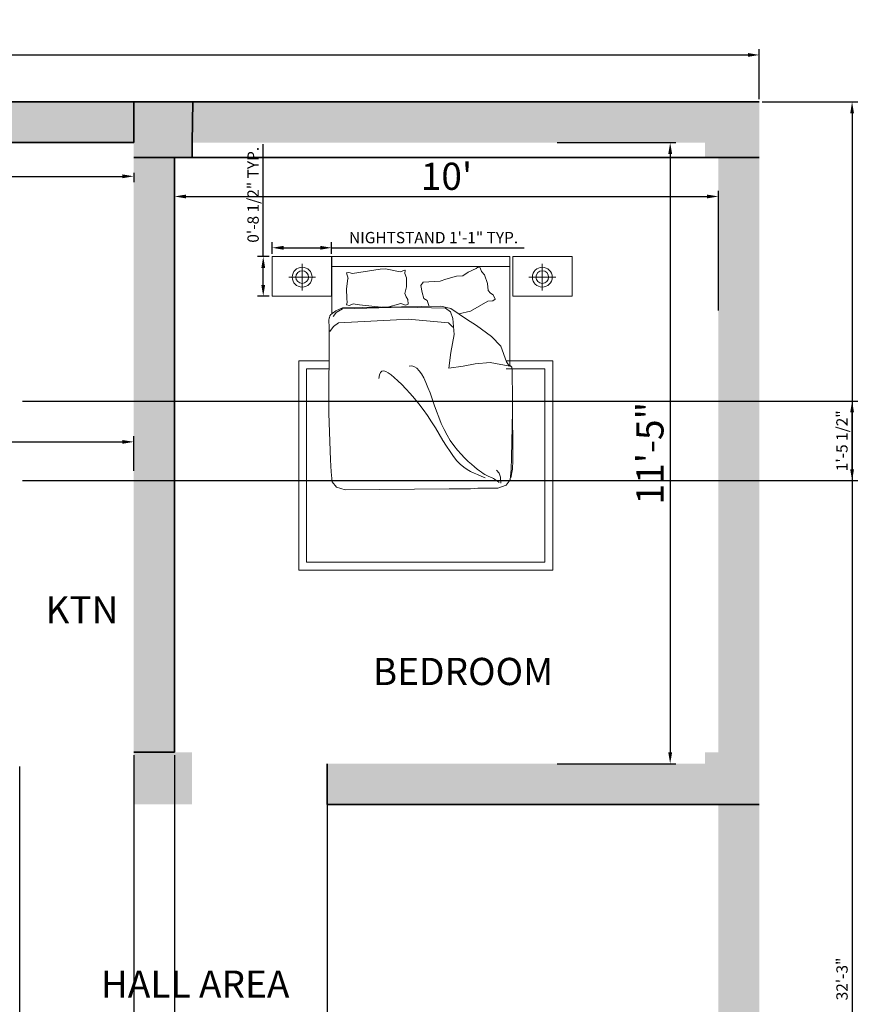
# Model space of a CAD drawing. Units: inches. Extents: x 3025 to 3429, y 1771 to 2198.
# Tile 3 of 3: x 3244 to 3429, y 1981 to 2198. Entities that reach past the tile are written whole.
import ezdxf

# ---------------------------------------------------------------- set-up
doc = ezdxf.new("R2010")
doc.units = ezdxf.units.IN
for name, color, linetype, lineweight in [('A-ANNO-DIMS', 2, 'Continuous', 18), ('A-AREA-IDEN', 7, 'Continuous', 25), ('A-COLS', 7, 'Continuous', 35), ('A-FURN', 8, 'Continuous', 18), ('A-WALL', 7, 'Continuous', 35), ('A-WALL-PATT', 3, 'Continuous', 13)]:
    doc.layers.add(name, color=color, linetype=linetype, lineweight=lineweight)
doc.layers.add('A-COLS-PATT', color=18, linetype='Continuous', lineweight=13, true_color=0x000000)
doc.styles.get("Standard").update_dxf_attribs({"font": 'arial.ttf'})
doc.dimstyles.new('ISO-25', dxfattribs={"dimtxt": 2.5, "dimasz": 2.5, "dimexe": 1.25, "dimexo": 0.625, "dimtad": 1, "dimdec": 0, "dimlunit": 3, "dimtxsty": 'Standard', "dimcen": 2.5, "dimadec": 0, "dimazin": 0, "dimtfac": 1, "dimtdec": 0, "dimtmove": 0, "dimatfit": 3, "dimfxl": 1, "dimarcsym": 0})

# ---------------------------------------------------------------- blocks, each defined once
blk = doc.blocks.new('*D1')
at = {"layer": 'A-ANNO-DIMS', "color": 0, "lineweight": -2, "transparency": 16777216}
for p, q in [((3054.93, 2180.84), (3054.93, 2191.81)), ((3406.93, 2180.84), (3406.93, 2191.81)), ((3057.43, 2190.56), (3404.43, 2190.56))]:
    blk.add_line(p, q, dxfattribs=at)
at = {"layer": 'A-ANNO-DIMS', "color": 0, "transparency": 16777216}
for points in [[(3057.43, 2190.98), (3057.43, 2190.14), (3054.93, 2190.56)], [(3404.43, 2190.98), (3404.43, 2190.14), (3406.93, 2190.56)]]:
    blk.add_solid(points, dxfattribs=at)
at = {"layer": 'Defpoints', "color": 0, "transparency": 16777216}
for p in [(3406.93, 2190.56), (3054.93, 2180.21), (3406.93, 2180.21)]:
    blk.add_point(p, dxfattribs=at)
at = {"layer": 'A-ANNO-DIMS', "color": 0, "transparency": 16777216, "insert": (3230.93, 2194.25), "char_height": 6, "attachment_point": 5}
blk.add_mtext('29\'-4"', dxfattribs=at)
blk = doc.blocks.new('*D9')
at = {"layer": 'A-ANNO-DIMS', "color": 0, "lineweight": -2, "transparency": 16777216}
for p, q in [((3192.93, 2164.54), (3192.93, 2162.53)), ((3195.43, 2163.78), (3266.43, 2163.78)), ((3268.93, 2164.54), (3268.93, 2162.53))]:
    blk.add_line(p, q, dxfattribs=at)
at = {"layer": 'A-ANNO-DIMS', "color": 0, "transparency": 16777216}
for points in [[(3195.43, 2164.2), (3195.43, 2163.37), (3192.93, 2163.78)], [(3266.43, 2164.2), (3266.43, 2163.37), (3268.93, 2163.78)]]:
    blk.add_solid(points, dxfattribs=at)
at = {"layer": 'Defpoints', "color": 0, "transparency": 16777216}
for p in [(3192.93, 2165.16), (3268.93, 2165.16), (3268.93, 2163.78)]:
    blk.add_point(p, dxfattribs=at)
at = {"layer": 'A-ANNO-DIMS', "color": 0, "transparency": 16777216, "insert": (3230.93, 2167.47), "char_height": 6, "attachment_point": 5}
blk.add_mtext('6\'-4"', dxfattribs=at)
blk = doc.blocks.new('*D10')
at = {"layer": 'A-ANNO-DIMS', "color": 0, "lineweight": -2, "transparency": 16777216}
for p, q in [((3277.93, 2134.19), (3277.93, 2160.59)), ((3280.43, 2159.34), (3395.43, 2159.34)), ((3397.93, 2134.19), (3397.93, 2160.59))]:
    blk.add_line(p, q, dxfattribs=at)
at = {"layer": 'A-ANNO-DIMS', "color": 0, "transparency": 16777216}
for points in [[(3280.43, 2159.75), (3280.43, 2158.92), (3277.93, 2159.34)], [(3395.43, 2159.75), (3395.43, 2158.92), (3397.93, 2159.34)]]:
    blk.add_solid(points, dxfattribs=at)
at = {"layer": 'Defpoints', "color": 0, "transparency": 16777216}
for p in [(3397.93, 2159.34), (3277.93, 2133.56), (3397.93, 2133.56)]:
    blk.add_point(p, dxfattribs=at)
at = {"layer": 'A-ANNO-DIMS', "color": 0, "transparency": 16777216, "insert": (3337.93, 2163.02), "char_height": 6, "attachment_point": 5}
blk.add_mtext("10'", dxfattribs=at)
blk = doc.blocks.new('*D13')
at = {"layer": 'A-ANNO-DIMS', "color": 0, "lineweight": -2, "transparency": 16777216}
for p, q in [((3362.35, 2171.21), (3388.54, 2171.21)), ((3387.29, 2168.71), (3387.29, 2036.71)), ((3362.35, 2034.21), (3388.54, 2034.21))]:
    blk.add_line(p, q, dxfattribs=at)
at = {"layer": 'A-ANNO-DIMS', "color": 0, "transparency": 16777216}
for points in [[(3386.87, 2168.71), (3387.71, 2168.71), (3387.29, 2171.21)], [(3386.87, 2036.71), (3387.71, 2036.71), (3387.29, 2034.21)]]:
    blk.add_solid(points, dxfattribs=at)
at = {"layer": 'Defpoints', "color": 0, "transparency": 16777216}
for p in [(3361.73, 2171.21), (3361.73, 2034.21), (3387.29, 2034.21)]:
    blk.add_point(p, dxfattribs=at)
at = {"layer": 'A-ANNO-DIMS', "color": 0, "transparency": 16777216, "insert": (3383.6, 2102.71), "char_height": 6, "attachment_point": 5, "rotation": 90}
blk.add_mtext('11\'-5"', dxfattribs=at)
blk = doc.blocks.new('*D15')
at = {"layer": 'A-ANNO-DIMS', "color": 0, "lineweight": -2, "transparency": 16777216}
for p, q in [((3192.93, 2097.44), (3192.93, 2106.45)), ((3195.43, 2105.2), (3266.43, 2105.2)), ((3268.93, 2098.84), (3268.93, 2106.45))]:
    blk.add_line(p, q, dxfattribs=at)
at = {"layer": 'A-ANNO-DIMS', "color": 0, "transparency": 16777216}
for points in [[(3195.43, 2105.61), (3195.43, 2104.78), (3192.93, 2105.2)], [(3266.43, 2105.61), (3266.43, 2104.78), (3268.93, 2105.2)]]:
    blk.add_solid(points, dxfattribs=at)
at = {"layer": 'Defpoints', "color": 0, "transparency": 16777216}
for p in [(3268.93, 2105.2), (3192.93, 2096.82), (3268.93, 2098.21)]:
    blk.add_point(p, dxfattribs=at)
at = {"layer": 'A-ANNO-DIMS', "color": 0, "transparency": 16777216, "insert": (3230.93, 2108.89), "char_height": 6, "attachment_point": 5}
blk.add_mtext('6\'-4"', dxfattribs=at)
blk = doc.blocks.new('NIGHTSTAND-13IN')
for p, q in [((6.62, 7.19), (6.62, 1.25)), ((3.65, 4.22), (9.59, 4.22))]:
    blk.add_line(p, q)
blk.add_lwpolyline([(0, 0), (13.1, 0), (13.1, 8.74), (0, 8.74)], close=True)
for radius in [2.19, 1.4]:
    blk.add_circle((6.62, 4.22), radius)
blk = doc.blocks.new('*D25')
at = {"layer": 'A-ANNO-DIMS', "color": 0, "lineweight": -2, "transparency": 16777216}
for p, q in [((3299.46, 2146.68), (3299.46, 2149.27)), ((3312.56, 2146.68), (3312.56, 2149.27)), ((3301.96, 2148.02), (3310.06, 2148.02)), ((3312.56, 2148.02), (3355.1, 2148.02))]:
    blk.add_line(p, q, dxfattribs=at)
at = {"layer": 'A-ANNO-DIMS', "color": 0, "transparency": 16777216}
for points in [[(3301.96, 2148.44), (3301.96, 2147.6), (3299.46, 2148.02)], [(3310.06, 2148.44), (3310.06, 2147.6), (3312.56, 2148.02)]]:
    blk.add_solid(points, dxfattribs=at)
at = {"layer": 'Defpoints', "color": 0, "transparency": 16777216}
for p in [(3312.56, 2148.02), (3299.46, 2146.06), (3312.56, 2146.06)]:
    blk.add_point(p, dxfattribs=at)
at = {"layer": 'A-ANNO-DIMS', "color": 0, "transparency": 16777216, "insert": (3335.08, 2149.94), "char_height": 2.5, "attachment_point": 5}
blk.add_mtext('NIGHTSTAND 1\'-1" TYP.', dxfattribs=at)
blk = doc.blocks.new('*D26')
at = {"layer": 'A-ANNO-DIMS', "color": 0, "lineweight": -2, "transparency": 16777216}
for p, q in [((3297.49, 2146.06), (3297.49, 2170.87)), ((3298.83, 2146.06), (3296.24, 2146.06)), ((3297.49, 2139.82), (3297.49, 2143.56)), ((3298.83, 2137.32), (3296.24, 2137.32))]:
    blk.add_line(p, q, dxfattribs=at)
at = {"layer": 'A-ANNO-DIMS', "color": 0, "transparency": 16777216}
for points in [[(3297.07, 2143.56), (3297.91, 2143.56), (3297.49, 2146.06)], [(3297.07, 2139.82), (3297.91, 2139.82), (3297.49, 2137.32)]]:
    blk.add_solid(points, dxfattribs=at)
at = {"layer": 'Defpoints', "color": 0, "transparency": 16777216}
for p in [(3297.49, 2146.06), (3299.46, 2146.06), (3299.46, 2137.32)]:
    blk.add_point(p, dxfattribs=at)
at = {"layer": 'A-ANNO-DIMS', "color": 0, "transparency": 16777216, "insert": (3295.57, 2159.71), "char_height": 2.5, "attachment_point": 5, "rotation": 90}
blk.add_mtext('0\'-8 1/2" TYP.', dxfattribs=at)
blk = doc.blocks.new('*D29')
at = {"layer": 'A-ANNO-DIMS', "color": 0, "lineweight": -2, "transparency": 16777216}
for p, q in [((3407.56, 2180.21), (3428.68, 2180.21)), ((3427.43, 2177.71), (3427.43, 1795.71)), ((3279.71, 1793.21), (3428.68, 1793.21))]:
    blk.add_line(p, q, dxfattribs=at)
at = {"layer": 'A-ANNO-DIMS', "color": 0, "transparency": 16777216}
for points in [[(3427.02, 2177.71), (3427.85, 2177.71), (3427.43, 2180.21)], [(3427.02, 1795.71), (3427.85, 1795.71), (3427.43, 1793.21)]]:
    blk.add_solid(points, dxfattribs=at)
at = {"layer": 'Defpoints', "color": 0, "transparency": 16777216}
for p in [(3406.93, 2180.21), (3279.09, 1793.21), (3427.43, 1793.21)]:
    blk.add_point(p, dxfattribs=at)
at = {"layer": 'A-ANNO-DIMS', "color": 0, "transparency": 16777216, "insert": (3425.53, 1986.71), "char_height": 2.5, "attachment_point": 5, "rotation": 90}
blk.add_mtext('32\'-3"', dxfattribs=at)
blk = doc.blocks.new('*D35')
at = {"layer": 'A-ANNO-DIMS', "color": 0, "lineweight": -2, "transparency": 16777216}
for p, q in [((3268.93, 2036.1), (3268.93, 1771.46)), ((3243.74, 2033.59), (3243.74, 1771.46)), ((3246.24, 1772.71), (3266.43, 1772.71))]:
    blk.add_line(p, q, dxfattribs=at)
at = {"layer": 'A-ANNO-DIMS', "color": 0, "transparency": 16777216}
for points in [[(3246.24, 1773.13), (3246.24, 1772.3), (3243.74, 1772.71)], [(3266.43, 1773.13), (3266.43, 1772.3), (3268.93, 1772.71)]]:
    blk.add_solid(points, dxfattribs=at)
at = {"layer": 'Defpoints', "color": 0, "transparency": 16777216}
for p in [(3268.93, 2036.73), (3243.74, 2034.21), (3268.93, 1772.71)]:
    blk.add_point(p, dxfattribs=at)
at = {"layer": 'A-ANNO-DIMS', "color": 0, "transparency": 16777216, "insert": (3256.34, 1774.59), "char_height": 2.5, "attachment_point": 5}
blk.add_mtext('2\'-1"', dxfattribs=at)
blk = doc.blocks.new('*D36')
at = {"layer": 'A-ANNO-DIMS', "color": 0, "lineweight": -2, "transparency": 16777216}
for p, q in [((3277.93, 2036.1), (3277.93, 1771.46)), ((3311.62, 2033.59), (3311.62, 1771.46)), ((3280.43, 1772.71), (3309.12, 1772.71))]:
    blk.add_line(p, q, dxfattribs=at)
at = {"layer": 'A-ANNO-DIMS', "color": 0, "transparency": 16777216}
for points in [[(3280.43, 1773.13), (3280.43, 1772.3), (3277.93, 1772.71)], [(3309.12, 1773.13), (3309.12, 1772.3), (3311.62, 1772.71)]]:
    blk.add_solid(points, dxfattribs=at)
at = {"layer": 'Defpoints', "color": 0, "transparency": 16777216}
for p in [(3277.93, 2036.73), (3311.62, 2034.21), (3311.62, 1772.71)]:
    blk.add_point(p, dxfattribs=at)
at = {"layer": 'A-ANNO-DIMS', "color": 0, "transparency": 16777216, "insert": (3294.78, 1774.63), "char_height": 2.5, "attachment_point": 5}
blk.add_mtext('2\'-9 1/2"', dxfattribs=at)
blk = doc.blocks.new('*D41')
at = {"layer": 'A-ANNO-DIMS', "color": 0, "lineweight": -2, "transparency": 16777216}
for p, q in [((3244.37, 2114.21), (3428.68, 2114.21)), ((3427.43, 2099.16), (3427.43, 2111.71)), ((3244.37, 2096.66), (3428.68, 2096.66))]:
    blk.add_line(p, q, dxfattribs=at)
at = {"layer": 'A-ANNO-DIMS', "color": 0, "transparency": 16777216}
for points in [[(3427.02, 2111.71), (3427.85, 2111.71), (3427.43, 2114.21)], [(3427.02, 2099.16), (3427.85, 2099.16), (3427.43, 2096.66)]]:
    blk.add_solid(points, dxfattribs=at)
at = {"layer": 'Defpoints', "color": 0, "transparency": 16777216}
for p in [(3243.74, 2114.21), (3427.43, 2114.21), (3243.74, 2096.66)]:
    blk.add_point(p, dxfattribs=at)
at = {"layer": 'A-ANNO-DIMS', "color": 0, "transparency": 16777216, "insert": (3425.52, 2105.44), "char_height": 2.5, "attachment_point": 5, "rotation": 90}
blk.add_mtext('1\'-5 1/2"', dxfattribs=at)

msp = doc.modelspace()

# ---------------------------------------------------------------- hatches: boundary and pattern name
at = {"layer": 'A-COLS-PATT'}
h = msp.add_hatch(color=256, dxfattribs=at)
h.dxf.hatch_style = 1
h.paths.add_polyline_path([(3281.8, 2036.73), (3277.93, 2036.73), (3268.93, 2036.73), (3268.93, 2025.21), (3277.93, 2025.21), (3281.8, 2025.21), (3281.8, 2034.21)])
h.paths.add_polyline_path([(3281.8, 2180.21), (3268.93, 2180.21), (3268.93, 2171.21), (3268.93, 2167.95), (3281.8, 2167.95)])
h = msp.add_hatch(color=256, dxfattribs=at)
h.dxf.hatch_style = 1
h.paths.add_polyline_path([(3397.93, 2036.73), (3395, 2036.73), (3395, 2034.21), (3397.93, 2034.21)])
h.paths.add_polyline_path([(3406.93, 2180.21), (3395, 2180.21), (3395, 2171.21), (3397.93, 2171.21), (3397.93, 2167.95), (3406.93, 2167.95)])
h.paths.add_polyline_path([(3397.93, 2171.21), (3395, 2171.21), (3395, 2167.95), (3397.93, 2167.95)], flags=17)
h = msp.add_hatch(color=256, dxfattribs=at)
h.dxf.hatch_style = 1
h.paths.add_polyline_path([(3406.93, 2036.73), (3397.93, 2036.73), (3397.93, 2034.21), (3395, 2034.21), (3395, 2025.21), (3397.93, 2025.21), (3406.93, 2025.21)])
at = {"layer": 'A-WALL-PATT'}
h = msp.add_hatch(color=256, dxfattribs=at)
h.dxf.hatch_style = 1
h.paths.add_polyline_path([(3268.93, 2180.21), (3192.93, 2180.21), (3192.93, 2171.21), (3268.93, 2171.21)])
h = msp.add_hatch(color=256, dxfattribs=at)
h.dxf.hatch_style = 1
h.paths.add_polyline_path([(3395, 2180.21), (3281.94, 2180.21), (3281.8, 2171.21), (3395, 2171.21)])
h.paths.add_polyline_path([(3406.93, 2167.95), (3397.93, 2167.95), (3397.93, 2036.73), (3406.93, 2036.73)])
h.paths.add_polyline_path([(3395, 2034.21), (3311.62, 2034.21), (3311.62, 2025.21), (3395, 2025.21)])
h = msp.add_hatch(color=256, dxfattribs=at)
h.dxf.hatch_style = 1
h.paths.add_polyline_path([(3277.93, 2167.95), (3268.93, 2167.95), (3268.93, 2036.73), (3277.93, 2036.73)])
h = msp.add_hatch(color=256, dxfattribs=at)
h.dxf.hatch_style = 1
h.paths.add_polyline_path([(3406.93, 1823.21), (3397.93, 1823.21), (3397.93, 1812.21), (3319.93, 1812.21), (3319.93, 1823.21), (3310.93, 1823.21), (3310.93, 1803.21), (3406.93, 1803.21)])
h.paths.add_polyline_path([(3406.93, 1952.09), (3397.93, 1952.09), (3397.93, 1835.41), (3406.93, 1835.41)])
h.paths.add_polyline_path([(3406.93, 2025.21), (3397.93, 2025.21), (3397.93, 1963.51), (3406.93, 1963.51)])

# ---------------------------------------------------------------- linework, layer by layer
at = {"layer": 'A-COLS'}
for p, q in [((3268.93, 2171.21), (3268.93, 2180.21)), ((3281.94, 2180.21), (3281.8, 2171.21)), ((3281.8, 2167.95), (3281.8, 2171.21)), ((3277.93, 2167.95), (3268.93, 2167.95)), ((3277.93, 2167.95), (3281.8, 2167.95)), ((3277.93, 2036.73), (3268.93, 2036.73)), ((3397.93, 2025.21), (3406.93, 2025.21))]:
    msp.add_line(p, q, dxfattribs=at)
at = {"layer": 'A-FURN'}
for p, q in [((3312.61, 2133.42), (3312.61, 2146.06)), ((3316.23, 2141.25), (3315.89, 2142.52)), ((3324.49, 2143.41), (3323.3, 2143.28)), ((3327.71, 2142.74), (3324.49, 2143.41)), ((3328.71, 2143.11), (3327.71, 2142.74)), ((3328.8, 2143.08), (3328.71, 2143.11)), ((3328.8, 2143.08), (3328.73, 2142.35)), ((3328.8, 2143.08), (3328.73, 2142.35)), ((3328.73, 2142.35), (3329.12, 2141.4)), ((3337.75, 2141.1), (3340.11, 2141.74)), ((3340.11, 2141.74), (3341.5, 2141.85)), ((3341.5, 2141.85), (3342.72, 2142.67)), ((3341.5, 2141.85), (3342.72, 2142.67)), ((3342.72, 2142.67), (3344.46, 2143.48)), ((3345.63, 2142.8), (3346.33, 2142.04)), ((3346.33, 2142.04), (3346.99, 2140.14)), ((3329.12, 2141.4), (3329.11, 2139.39)), ((3332.8, 2140.41), (3336.5, 2140.63)), ((3336.5, 2140.63), (3337.75, 2141.1)), ((3346.99, 2140.14), (3347.16, 2138.62)), ((3329.11, 2139.39), (3328.75, 2137.9)), ((3328.75, 2137.9), (3329, 2137.19)), ((3347.16, 2138.62), (3347.63, 2138.03)), ((3347.63, 2138.03), (3348.24, 2137.65)), ((3348.24, 2137.65), (3348.65, 2136.68)), ((3327.87, 2135.69), (3324.68, 2134.87)), ((3328.88, 2135.37), (3327.87, 2135.69)), ((3329.5, 2135.57), (3328.88, 2135.37)), ((3329, 2137.19), (3329.43, 2136.62)), ((3329.43, 2136.62), (3329.5, 2135.57)), ((3347.08, 2136.24), (3343.21, 2134.07)), ((3348.14, 2136.28), (3347.08, 2136.24)), ((3348.65, 2136.68), (3348.14, 2136.28)), ((3312.06, 2132.55), (3312, 2131.94)), ((3312, 2131.94), (3312.02, 2130.51)), ((3312.02, 2130.51), (3311.94, 2111.48)), ((3351.87, 2121.93), (3351.95, 2121.97)), ((3352.46, 2114.61), (3352.39, 2120.78)), ((3352.6, 2101.09), (3352.46, 2114.61)), ((3311.94, 2111.48), (3312.35, 2101.27)), ((3352.5, 2111.96), (3352.24, 2101.74)), ((3312.35, 2101.27), (3312.49, 2098.6)), ((3352.24, 2101.74), (3352.18, 2099.07)), ((3352.48, 2099.21), (3352.6, 2101.09)), ((3312.49, 2098.6), (3312.73, 2096.4)), ((3349.58, 2098.31), (3348.94, 2098.99)), ((3349.87, 2097.42), (3349.58, 2098.31)), ((3352.18, 2099.07), (3352, 2096.86)), ((3352.11, 2097.26), (3352.48, 2099.21)), ((3312.73, 2096.4), (3313.69, 2095.24)), ((3349.93, 2096.12), (3349.87, 2097.42)), ((3352, 2096.86), (3351.08, 2095.67)), ((3313.69, 2095.24), (3315.56, 2094.61)), ((3338.51, 2094.86), (3315.56, 2094.61)), ((3338.51, 2094.86), (3343.19, 2094.86)), ((3343.19, 2094.86), (3344.85, 2094.98)), ((3344.85, 2094.98), (3349.23, 2094.98)), ((3351.08, 2095.67), (3349.23, 2094.98))]:
    msp.add_line(p, q, dxfattribs=at)
for points in [[(3312.61, 2146.06), (3351.94, 2146.06), (3351.94, 2122)], [(3351.94, 2143.87), (3312.61, 2143.87)], [(3323.3, 2143.28), (3318.55, 2142.57), (3317.17, 2142.33), (3316.35, 2142.6), (3315.89, 2142.52)], [(3345.63, 2142.8), (3345.38, 2143.6), (3344.86, 2143.77), (3344.46, 2143.48)], [(3323.49, 2134.95), (3318.7, 2135.45), (3317.32, 2135.62), (3316.51, 2135.32), (3315.84, 2135.41), (3316.02, 2135.94), (3315.91, 2136.85), (3315.88, 2138.95), (3316.18, 2141.25)], [(3332.8, 2140.41), (3332.3, 2139.69), (3332.54, 2138.17), (3332.9, 2136.83), (3333.63, 2136.41), (3334.06, 2135.32), (3334.06, 2135.11)], [(3312.08, 2132.59), (3312.2, 2133), (3312.39, 2133.31), (3312.61, 2133.42), (3312.87, 2133.64), (3312.9, 2133.66)], [(3351.94, 2121.91), (3347.53, 2122.68), (3344.28, 2122.44), (3341.62, 2121.9), (3338.47, 2121.46), (3338.89, 2124.9), (3339.6, 2128.9), (3339.29, 2132.44), (3338.83, 2133.87), (3337.68, 2134.69), (3328.36, 2134.94), (3314.96, 2134.54), (3313.59, 2133.73), (3313.01, 2132.93), (3312.93, 2132.85)], [(3312.94, 2133.65), (3313.48, 2134.12), (3314.95, 2134.74), (3336.68, 2135.16), (3338.86, 2134.6), (3342.35, 2132.29), (3344.55, 2130.84), (3347.84, 2128.42), (3349.94, 2126.28), (3351.18, 2122.84), (3351.79, 2121.94)], [(3343.21, 2134.07), (3340.63, 2133.43)], [(3339.34, 2130.48), (3338.35, 2131.49), (3329.48, 2132.24), (3326.9, 2132.09), (3314.06, 2131.45), (3312.97, 2130.63), (3312.16, 2129.54)], [(3351.09, 2123.08), (3361.38, 2123.08), (3361.38, 2076.91), (3305.31, 2076.91), (3305.31, 2123.08), (3311.99, 2123.08)], [(3351.09, 2121.34), (3359.63, 2121.34), (3359.63, 2078.66), (3307.05, 2078.66), (3307.05, 2121.34), (3311.99, 2121.34)], [(3346.44, 2097.29), (3345.61, 2097.66), (3344.8, 2097.99), (3344, 2098.33), (3343.23, 2098.69), (3342.47, 2099.12), (3341.72, 2099.63), (3340.97, 2100.25), (3340.22, 2101.03), (3339.47, 2101.96), (3338.71, 2103.04), (3337.94, 2104.24), (3337.15, 2105.53), (3336.34, 2106.88), (3335.51, 2108.27), (3334.64, 2109.65), (3333.74, 2111.02), (3332.8, 2112.33), (3331.84, 2113.59), (3330.86, 2114.77), (3329.9, 2115.88), (3328.95, 2116.91), (3328.05, 2117.84), (3327.19, 2118.67), (3326.41, 2119.38), (3325.7, 2119.98), (3325.08, 2120.44), (3324.54, 2120.74), (3324.07, 2120.86), (3323.69, 2120.79), (3323.38, 2120.5), (3323.15, 2119.97), (3322.99, 2119.19)], [(3349.55, 2096.26), (3349.18, 2096.54), (3348.85, 2096.77), (3348.55, 2096.95), (3348.27, 2097.11), (3348, 2097.25), (3347.75, 2097.36), (3347.5, 2097.48), (3347.25, 2097.59), (3346.98, 2097.71), (3346.7, 2097.85), (3346.39, 2098.02), (3346.04, 2098.23), (3345.64, 2098.49), (3345.2, 2098.81), (3344.68, 2099.21), (3344.1, 2099.68), (3343.43, 2100.25), (3342.71, 2100.9), (3341.93, 2101.65), (3341.14, 2102.48), (3340.33, 2103.4), (3339.53, 2104.41), (3338.77, 2105.51), (3338.05, 2106.69), (3337.39, 2107.95), (3336.78, 2109.27), (3336.23, 2110.64), (3335.71, 2112.01), (3335.22, 2113.38), (3334.76, 2114.72), (3334.3, 2116.01), (3333.84, 2117.22), (3333.38, 2118.33), (3332.9, 2119.32), (3332.41, 2120.18), (3331.91, 2120.89), (3331.39, 2121.44), (3330.84, 2121.79), (3330.27, 2121.94), (3329.67, 2121.88)], [(3352.39, 2120.84), (3352.33, 2121.69), (3352.08, 2121.94), (3351.94, 2122)]]:
    msp.add_lwpolyline(points, dxfattribs=at)
at = {"layer": 'A-WALL'}
for p, q in [((3054.93, 2180.21), (3406.93, 2180.21)), ((3192.93, 2171.21), (3268.93, 2171.21)), ((3277.93, 2167.95), (3277.93, 2036.73)), ((3281.8, 2167.95), (3406.93, 2167.95)), ((3311.62, 2034.21), (3311.62, 2025.21)), ((3311.62, 2025.21), (3397.93, 2025.21))]:
    msp.add_line(p, q, dxfattribs=at)

# ---------------------------------------------------------------- block references
at = {"layer": 'A-FURN'}
msp.add_blockref('NIGHTSTAND-13IN', (3299.46, 2137.32), dxfattribs=at)
at = {"layer": 'A-FURN', "extrusion": (0, 0, -1), "zscale": -1}
msp.add_blockref('NIGHTSTAND-13IN', (-3365.69, 2137.32), dxfattribs=at)

# ---------------------------------------------------------------- texts
at = {"layer": 'A-AREA-IDEN', "char_height": 6, "attachment_point": 1}
for s, insert in [('KTN', (3249.43, 2071.16)), ('BEDROOM', (3321.66, 2057.55)), ('HALL AREA', (3261.64, 1988.57))]:
    msp.add_mtext(s, dxfattribs=dict(at, insert=insert))

# ---------------------------------------------------------------- dimensions: what is measured, and where the dimension line sits
at = {"layer": 'A-ANNO-DIMS'}
for base, p1, p2, override, picture, middle in [((3406.93, 2190.56), (3054.93, 2180.21), (3406.93, 2180.21), {"dimtxt": 6, "dimclrd": 0, "dimclre": 0, "dimclrt": 0}, '*D1', (3230.93, 2194.25)), ((3268.93, 2163.78), (3192.93, 2165.16), (3268.93, 2165.16), {"dimtxt": 6, "dimclrd": 0, "dimclre": 0, "dimclrt": 0}, '*D9', (3230.93, 2167.47)), ((3397.93, 2159.34), (3277.93, 2133.56), (3397.93, 2133.56), {"dimtxt": 6, "dimclrd": 0, "dimclre": 0, "dimclrt": 0}, '*D10', (3337.93, 2163.02)), ((3268.93, 2105.2), (3192.93, 2096.82), (3268.93, 2098.21), {"dimtxt": 6, "dimclrd": 0, "dimclre": 0, "dimclrt": 0}, '*D15', (3230.93, 2108.89)), ((3268.93, 1772.71), (3243.74, 2034.21), (3268.93, 2036.73), {"dimdec": 1, "dimlfac": 1, "dimrnd": 0, "dimzin": 1, "dimdsep": 46, "dimlunit": 4, "dimfrac": 2}, '*D35', (3256.34, 1774.59)), ((3311.62, 1772.71), (3277.93, 2036.73), (3311.62, 2034.21), {"dimdec": 1, "dimlfac": 1, "dimrnd": 0, "dimzin": 1, "dimdsep": 46, "dimlunit": 4, "dimfrac": 2}, '*D36', (3294.78, 1774.63))]:
    dim = msp.add_linear_dim(base=base, p1=p1, p2=p2, dimstyle='ISO-25', override=override, dxfattribs=at)
    dim.commit()
    dim.dimension.update_dxf_attribs({"geometry": picture, "text_midpoint": middle})
for base, p1, p2, override, picture, middle in [((3427.43, 1793.21), (3406.93, 2180.21), (3279.09, 1793.21), {"dimdec": 1, "dimlfac": 1, "dimrnd": 0, "dimzin": 1, "dimdsep": 46, "dimlunit": 4, "dimfrac": 2}, '*D29', (3425.53, 1986.71)), ((3387.29, 2034.21), (3361.73, 2171.21), (3361.73, 2034.21), {"dimtxt": 6, "dimclrd": 0, "dimclre": 0, "dimclrt": 0}, '*D13', (3383.6, 2102.71)), ((3427.4341, 2114.2132), (3243.7445, 2096.658), (3243.7445, 2114.2132), {"dimdec": 1, "dimlfac": 1, "dimrnd": 0, "dimzin": 1, "dimdsep": 46, "dimlunit": 4, "dimfrac": 2}, '*D41', (3425.5165, 2105.4356))]:
    dim = msp.add_linear_dim(base=base, p1=p1, p2=p2, angle=90, dimstyle='ISO-25', override=override, dxfattribs=at)
    dim.commit()
    dim.dimension.update_dxf_attribs({"geometry": picture, "text_midpoint": middle})
dim = msp.add_linear_dim(base=(3297.49, 2146.06), p1=(3299.46, 2137.32), p2=(3299.46, 2146.06), angle=90, text='<> TYP.', dimstyle='ISO-25', override={"dimdec": 1, "dimlfac": 1, "dimrnd": 0, "dimzin": 1, "dimdsep": 46, "dimlunit": 4, "dimfrac": 2}, dxfattribs=at)
dim.commit()
dim.dimension.update_dxf_attribs({"geometry": '*D26', "text_midpoint": (3295.57, 2159.71)})
dim = msp.add_linear_dim(base=(3312.56, 2148.02), p1=(3299.46, 2146.06), p2=(3312.56, 2146.06), text='NIGHTSTAND <> TYP.', dimstyle='ISO-25', override={"dimdec": 1, "dimlfac": 1, "dimrnd": 0, "dimzin": 1, "dimdsep": 46, "dimlunit": 4, "dimfrac": 2}, dxfattribs=at)
dim.commit()
dim.dimension.update_dxf_attribs({"geometry": '*D25', "text_midpoint": (3335.08, 2149.94)})

doc.saveas('drawing.dxf')
